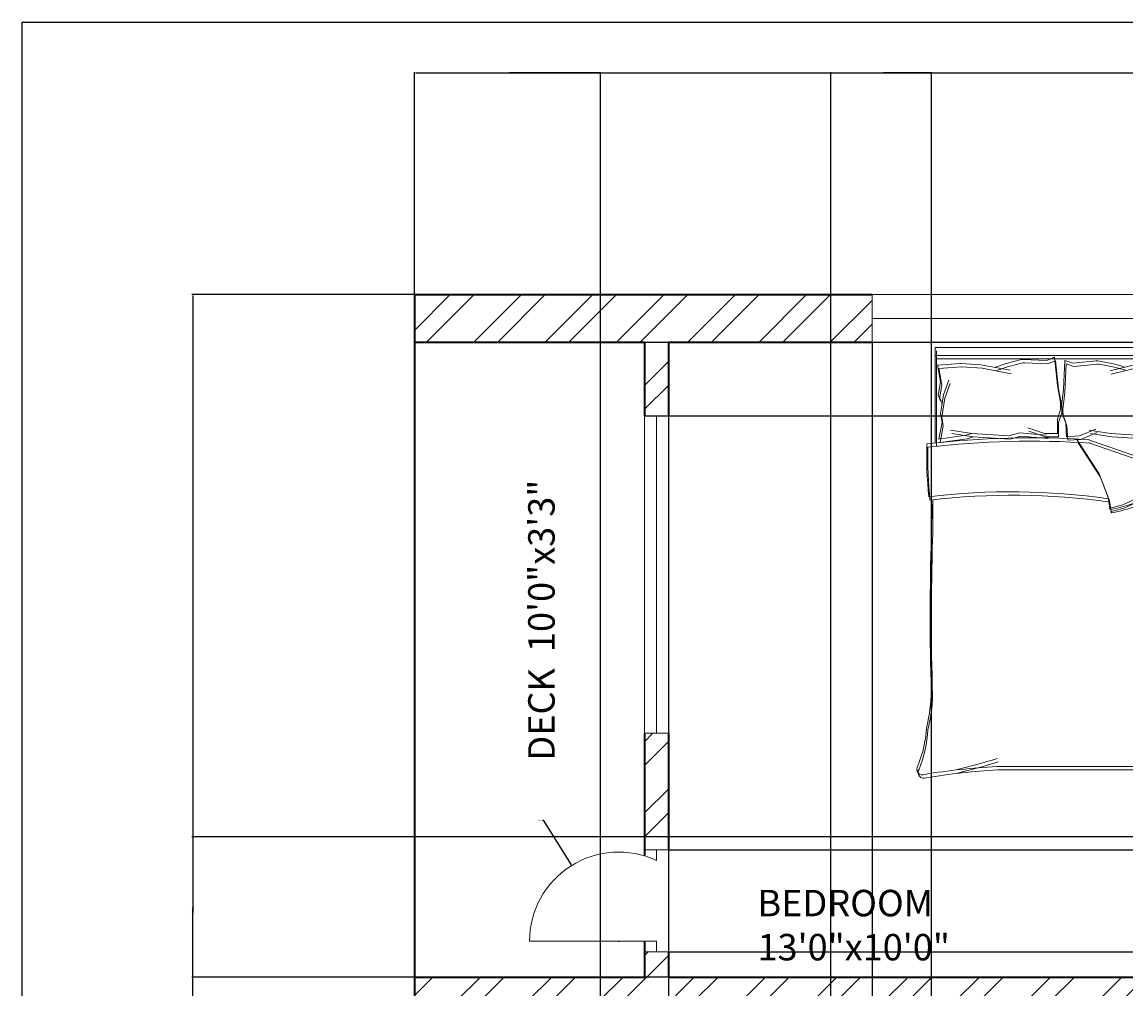
# Model space of a CAD drawing. Units: inches. Extents: x 1748 to 2382, y 1346 to 2284.
# Tile 20 of 26: x 1748 to 1956, y 2102 to 2284. Entities that reach past the tile are written whole.
import ezdxf

# ---------------------------------------------------------------- set-up
doc = ezdxf.new("R2010")
doc.units = ezdxf.units.IN
for name, color, linetype, lineweight in [('A-ANNO-DIMS', 2, 'Continuous', 18), ('A-ANNO-TTLB', 7, 'Continuous', 25), ('A-AREA-IDEN', 7, 'Continuous', 18), ('A-DOOR', 21, 'Continuous', 18), ('A-FURN', 8, 'Continuous', 13), ('A-GLAZ', 191, 'Continuous', 18), ('A-WALL', 7, 'Continuous', 35), ('A-WALL-PATT', 9, 'Continuous', 13)]:
    doc.layers.add(name, color=color, linetype=linetype, lineweight=lineweight)
doc.styles.get("Standard").update_dxf_attribs({"font": 'arial.ttf'})
doc.dimstyles.get("Standard").update_dxf_attribs({"dimtxt": 0.18, "dimasz": 0.18, "dimexe": 0.18, "dimexo": 0.0625, "dimgap": 0.09, "dimtad": 0, "dimtih": 1, "dimtoh": 1, "dimdec": 4, "dimzin": 0, "dimdsep": 46, "dimtxsty": 'Standard', "dimcen": 0.09, "dimadec": 0, "dimazin": 0, "dimtfac": 1, "dimtdec": 4, "dimtofl": 0, "dimtmove": 0, "dimatfit": 3, "dimfxl": 1, "dimtolj": 1, "dimtzin": 0, "dimarcsym": 0})

# ---------------------------------------------------------------- blocks, each defined once
blk = doc.blocks.new('BED-DOUBLE')
for p, q in [((3.48, 63.33), (3.48, 81.44)), ((3.48, 63.33), (3.48, 81.44)), ((3.48, 81.44), (51.49, 81.44)), ((51.27, 81.44), (51.27, 54.83)), ((51.27, 81.44), (51.27, 54.83)), ((51.49, 81.44), (51.49, 80.8)), ((3.48, 79.91), (51.27, 79.91)), ((3.48, 79.91), (51.27, 79.91)), ((3.7, 62.69), (3.7, 80.8)), ((3.7, 62.69), (3.7, 80.8)), ((24.54, 78.99), (25.98, 79.57)), ((24.54, 78.99), (25.98, 79.57)), ((25.98, 79.57), (26.56, 74.22)), ((25.98, 79.57), (26.56, 74.22)), ((51.49, 80.8), (51.49, 54.19)), ((51.49, 80.8), (51.49, 54.19)), ((3.7, 79.27), (51.49, 79.27)), ((3.7, 79.27), (51.49, 79.27)), ((3.89, 78.13), (4.47, 74.95)), ((3.9, 78.11), (8.18, 78.43)), ((3.9, 78.11), (8.18, 78.43)), ((3.9, 78.13), (4.47, 74.95)), ((4.12, 77.49), (4.7, 74.31)), ((4.12, 77.49), (4.7, 74.31)), ((4.13, 77.47), (8.41, 77.8)), ((4.13, 77.47), (8.41, 77.8)), ((8.18, 78.43), (8.29, 78.42)), ((8.18, 78.43), (8.28, 78.42)), ((8.28, 78.42), (12.11, 78.13)), ((8.29, 78.42), (12.11, 78.13)), ((8.41, 77.8), (8.51, 77.78)), ((8.41, 77.8), (8.51, 77.78)), ((8.51, 77.78), (12.34, 77.49)), ((8.51, 77.78), (12.34, 77.49)), ((12.11, 78.13), (17.6, 77.12)), ((12.11, 78.13), (17.6, 77.12)), ((12.34, 77.49), (17.83, 76.48)), ((12.34, 77.49), (17.83, 76.48)), ((14.86, 77.69), (16.88, 78.42)), ((14.86, 77.69), (16.88, 78.42)), ((15.08, 77.05), (17.11, 77.78)), ((15.08, 77.05), (17.11, 77.78)), ((16.88, 78.42), (19.77, 79.14)), ((16.88, 78.42), (19.77, 79.14)), ((17.11, 77.78), (20, 78.5)), ((17.11, 77.78), (20, 78.5)), ((19.77, 79.14), (20.09, 79.14)), ((19.77, 79.14), (20.09, 79.14)), ((20, 78.5), (20.32, 78.5)), ((20, 78.5), (20.32, 78.5)), ((20.09, 79.14), (24.54, 78.99)), ((20.09, 79.14), (24.54, 78.99)), ((20.32, 78.5), (24.77, 78.36)), ((20.32, 78.5), (24.77, 78.36)), ((24.77, 78.36), (26.21, 78.93)), ((24.77, 78.36), (26.21, 78.93)), ((26.21, 78.93), (26.79, 73.58)), ((26.21, 78.93), (26.79, 73.58)), ((27.98, 78.95), (27.73, 73.58)), ((27.98, 78.95), (27.73, 73.58)), ((28.21, 78.31), (27.96, 72.94)), ((28.21, 78.31), (27.96, 72.94)), ((29.46, 78.46), (27.98, 78.95)), ((29.46, 78.46), (27.98, 78.95)), ((29.68, 77.83), (28.21, 78.31)), ((29.68, 77.83), (28.21, 78.31)), ((33.88, 78.89), (29.46, 78.46)), ((33.88, 78.89), (29.46, 78.46)), ((34.11, 78.25), (29.68, 77.83)), ((34.11, 78.25), (29.68, 77.83)), ((34.21, 78.91), (33.88, 78.89)), ((34.2, 78.91), (33.88, 78.89)), ((34.43, 78.27), (34.11, 78.25)), ((34.43, 78.27), (34.11, 78.25)), ((37.14, 78.37), (34.2, 78.91)), ((37.14, 78.37), (34.21, 78.91)), ((37.36, 77.73), (34.43, 78.27)), ((37.36, 77.73), (34.43, 78.27)), ((41.91, 78.37), (36.5, 77.02)), ((41.91, 78.37), (36.5, 77.02)), ((42.14, 77.73), (36.72, 76.38)), ((42.14, 77.73), (36.72, 76.38)), ((39.2, 77.77), (37.14, 78.37)), ((39.2, 77.77), (37.14, 78.37)), ((39.43, 77.13), (37.36, 77.73)), ((39.43, 77.13), (37.36, 77.73)), ((45.71, 78.9), (41.91, 78.37)), ((45.71, 78.9), (41.91, 78.37)), ((45.94, 78.26), (42.14, 77.73)), ((45.94, 78.26), (42.14, 77.73)), ((50.11, 78.89), (44.71, 78.98)), ((44.71, 78.98), (45.71, 78.9)), ((50.11, 78.89), (44.71, 78.98)), ((44.71, 78.98), (45.71, 78.9)), ((50.34, 78.25), (44.94, 78.34)), ((44.94, 78.34), (45.94, 78.26)), ((50.34, 78.25), (44.94, 78.34)), ((44.94, 78.34), (45.94, 78.26)), ((50.11, 78.89), (49.73, 75.68)), ((50.11, 78.89), (49.73, 75.68)), ((50.34, 78.25), (49.96, 75.04)), ((50.34, 78.25), (49.96, 75.04)), ((5.05, 72.49), (6.06, 75.24)), ((5.05, 72.49), (6.06, 75.24)), ((49.31, 73.19), (48.13, 75.87)), ((49.31, 73.19), (48.13, 75.87)), ((49.54, 72.55), (48.36, 75.23)), ((49.54, 72.55), (48.36, 75.23)), ((49.73, 75.68), (50.33, 73.11)), ((49.73, 75.68), (50.33, 73.11)), ((4.47, 74.95), (4.04, 72.34)), ((4.47, 74.95), (4.04, 72.34)), ((4.7, 74.31), (4.27, 71.7)), ((4.7, 74.31), (4.27, 71.7)), ((5.28, 71.85), (6.29, 74.6)), ((5.28, 71.85), (6.29, 74.6)), ((26.56, 74.22), (27.14, 71.04)), ((26.56, 74.22), (27.14, 71.04)), ((26.79, 73.58), (27.37, 70.4)), ((26.79, 73.58), (27.37, 70.4)), ((27.73, 73.58), (27.35, 70.37)), ((27.73, 73.58), (27.36, 70.37)), ((50.11, 69.61), (49.31, 73.19)), ((50.11, 69.61), (49.31, 73.19)), ((50.33, 73.11), (49.81, 72.06)), ((50.33, 73.11), (49.81, 72.06)), ((49.96, 75.04), (50.56, 72.47)), ((49.96, 75.04), (50.56, 72.47)), ((4.04, 72.34), (4.62, 71.33)), ((4.04, 72.34), (4.62, 71.33)), ((4.27, 71.7), (4.85, 70.69)), ((4.27, 71.7), (4.85, 70.69)), ((4.47, 68.87), (5.05, 72.49)), ((4.47, 68.87), (5.05, 72.49)), ((4.7, 68.23), (5.28, 71.85)), ((4.7, 68.23), (5.28, 71.85)), ((27.14, 71.04), (27.14, 69.74)), ((27.14, 71.04), (27.14, 69.74)), ((27.96, 72.94), (27.58, 69.73)), ((27.96, 72.94), (27.58, 69.73)), ((50.34, 68.98), (49.54, 72.55)), ((50.34, 68.98), (49.54, 72.55)), ((50.56, 72.47), (50.04, 71.42)), ((50.56, 72.47), (50.04, 71.42)), ((4.76, 67.28), (4.47, 68.87)), ((4.76, 67.28), (4.47, 68.87)), ((27.14, 69.74), (26.56, 67.86)), ((27.14, 69.74), (26.56, 67.86)), ((27.37, 69.1), (26.79, 67.22)), ((27.37, 69.1), (26.79, 67.22)), ((27.35, 70.37), (27.44, 69.07)), ((27.36, 70.37), (27.44, 69.07)), ((27.37, 70.4), (27.37, 69.1)), ((27.37, 70.4), (27.37, 69.1)), ((27.44, 69.07), (28.13, 67.23)), ((27.44, 69.07), (28.13, 67.23)), ((27.58, 69.73), (27.66, 68.43)), ((27.58, 69.73), (27.66, 68.43)), ((49.92, 68.01), (50.11, 69.61)), ((49.92, 68.01), (50.11, 69.61)), ((50.15, 67.37), (50.34, 68.98)), ((50.15, 67.37), (50.34, 68.98)), ((4.18, 64.1), (4.76, 67.28)), ((4.18, 64.1), (4.76, 67.28)), ((4.99, 66.64), (4.7, 68.23)), ((4.99, 66.64), (4.7, 68.23)), ((26.56, 67.86), (26.56, 65.18)), ((26.56, 67.86), (26.56, 65.18)), ((26.79, 67.22), (26.79, 64.54)), ((26.79, 67.22), (26.79, 64.54)), ((27.66, 68.43), (28.36, 66.59)), ((27.66, 68.43), (28.36, 66.59)), ((28.13, 67.23), (28.3, 64.55)), ((28.13, 67.23), (28.3, 64.55)), ((50.7, 64.87), (49.92, 68.01)), ((50.7, 64.87), (49.92, 68.01)), ((50.93, 64.23), (50.15, 67.37)), ((50.93, 64.23), (50.15, 67.37)), ((9.28, 64.83), (4.18, 64.1)), ((9.28, 64.83), (4.18, 64.1)), ((4.41, 63.46), (4.99, 66.64)), ((4.41, 63.46), (4.99, 66.64)), ((6.38, 65.81), (10.41, 65.15)), ((6.38, 65.81), (10.41, 65.15)), ((6.61, 65.18), (10.64, 64.51)), ((6.61, 65.18), (10.64, 64.51)), ((10.41, 65.15), (9.28, 64.83)), ((10.41, 65.15), (9.28, 64.83)), ((10.41, 65.15), (17.42, 64.72)), ((10.41, 65.15), (17.42, 64.72)), ((17.42, 64.72), (19.38, 65.27)), ((17.42, 64.72), (19.38, 65.27)), ((19.38, 65.27), (24.52, 64.87)), ((19.38, 65.27), (24.52, 64.87)), ((24.1, 65.18), (20.96, 66.27)), ((24.1, 65.18), (20.96, 66.27)), ((24.33, 64.54), (21.19, 65.63)), ((24.33, 64.54), (21.19, 65.63)), ((26.56, 65.18), (24.1, 65.18)), ((26.56, 65.18), (24.1, 65.18)), ((28.3, 64.55), (30.75, 64.7)), ((28.3, 64.55), (30.75, 64.7)), ((28.36, 66.59), (28.53, 63.91)), ((28.36, 66.59), (28.53, 63.91)), ((30.75, 64.7), (33.82, 65.99)), ((30.75, 64.7), (33.82, 65.99)), ((30.98, 64.06), (34.05, 65.35)), ((30.98, 64.06), (34.05, 65.35)), ((32.56, 65.81), (36.6, 65.15)), ((32.56, 65.81), (36.6, 65.15)), ((32.79, 65.18), (36.83, 64.51)), ((32.79, 65.18), (36.82, 64.51)), ((36.6, 65.15), (43.61, 64.72)), ((36.6, 65.15), (43.61, 64.72)), ((43.61, 64.72), (45.57, 65.27)), ((43.61, 64.72), (45.57, 65.27)), ((45.57, 65.27), (50.7, 64.87)), ((45.57, 65.27), (50.7, 64.87)), ((9.51, 64.19), (4.41, 63.46)), ((9.51, 64.19), (4.41, 63.46)), ((10.64, 64.51), (9.51, 64.19)), ((10.64, 64.51), (9.51, 64.19)), ((10.64, 64.51), (17.65, 64.08)), ((10.64, 64.51), (17.65, 64.08)), ((17.65, 64.08), (19.61, 64.64)), ((17.65, 64.08), (19.61, 64.64)), ((19.61, 64.64), (24.74, 64.23)), ((19.61, 64.64), (24.74, 64.23)), ((26.79, 64.54), (24.33, 64.54)), ((26.79, 64.54), (24.33, 64.54)), ((28.53, 63.91), (30.98, 64.06)), ((28.53, 63.91), (30.98, 64.06)), ((30.26, 64.06), (34.45, 57.57)), ((30.26, 64.06), (34.45, 57.57)), ((30.49, 63.42), (34.68, 56.93)), ((30.49, 63.42), (34.68, 56.93)), ((40.64, 61.13), (32.31, 64.06)), ((40.64, 61.13), (32.31, 64.06)), ((40.87, 60.49), (32.53, 63.42)), ((40.87, 60.49), (32.53, 63.42)), ((36.82, 64.51), (43.83, 64.08)), ((36.83, 64.51), (43.83, 64.08)), ((43.83, 64.08), (45.8, 64.64)), ((43.83, 64.08), (45.79, 64.64)), ((45.79, 64.64), (50.93, 64.23)), ((45.8, 64.64), (50.93, 64.23)), ((46.22, 59.11), (40.64, 61.13)), ((46.22, 59.11), (40.64, 61.13)), ((46.45, 58.48), (40.87, 60.49)), ((46.45, 58.48), (40.87, 60.49)), ((49.16, 56.95), (46.22, 59.11)), ((49.16, 56.95), (46.22, 59.11)), ((49.39, 56.31), (46.45, 58.48)), ((49.39, 56.31), (46.45, 58.48)), ((34.45, 57.57), (36.15, 53.08)), ((34.45, 57.57), (36.15, 53.08)), ((34.68, 56.93), (36.38, 52.44)), ((34.68, 56.93), (36.38, 52.44)), ((52.87, 53.7), (49.16, 56.95)), ((52.87, 53.7), (49.16, 56.95)), ((53.1, 53.06), (49.39, 56.31)), ((53.1, 53.06), (49.39, 56.31)), ((36.15, 53.08), (36.46, 51.07)), ((36.15, 53.08), (36.46, 51.07)), ((36.38, 52.44), (36.69, 50.43)), ((36.38, 52.44), (36.69, 50.43)), ((38.94, 51.69), (40.95, 52.61)), ((38.94, 51.69), (40.95, 52.61)), ((40.95, 52.61), (44.36, 53.08)), ((40.95, 52.61), (44.36, 53.08)), ((41.18, 51.97), (44.59, 52.44)), ((41.18, 51.97), (44.59, 52.44)), ((44.36, 53.08), (48.23, 53.39)), ((44.36, 53.08), (48.23, 53.39)), ((44.59, 52.44), (48.46, 52.75)), ((44.59, 52.44), (48.46, 52.75)), ((48.23, 53.39), (51.33, 53.08)), ((48.23, 53.39), (51.33, 53.08)), ((48.46, 52.75), (51.56, 52.44)), ((48.46, 52.75), (51.56, 52.44)), ((51.33, 53.08), (52.87, 53.7)), ((51.33, 53.08), (52.87, 53.7)), ((51.56, 52.44), (53.1, 53.06)), ((51.56, 52.44), (53.1, 53.06)), ((52.95, 51.95), (52.87, 53.7, 3.87)), ((52.95, 51.95), (52.87, 53.7, 3.87)), ((53.18, 51.31), (53.1, 53.06, 3.87)), ((53.18, 51.31), (53.1, 53.06, 3.87)), ((36.46, 51.07), (38.94, 51.69)), ((36.46, 51.07), (38.94, 51.69)), ((36.69, 50.43), (39.17, 51.05)), ((36.69, 50.43), (39.17, 51.05)), ((39.17, 51.05), (41.18, 51.97)), ((39.17, 51.05), (41.18, 51.97)), ((15.06, 2.2), (39.68, 2.2)), ((15.06, 2.2), (39.68, 2.2)), ((15.29, 1.56), (39.91, 1.56)), ((15.29, 1.56), (39.91, 1.56))]:
    blk.add_line(p, q)
for centre, radius, start, end in [((85.16, 61.35), 83.31, 178.7218, 185.604), ((85.16, 61.35), 83.31, 178.7218, 185.604), ((21.36, -100.61), 164.97, 86.0865, 96.7821), ((21.36, -100.61), 164.97, 86.0865, 96.7821), ((21.59, -101.25), 164.97, 86.0865, 96.7821), ((21.59, -101.25), 164.97, 86.0865, 96.7821), ((85.39, 60.71), 83.31, 178.7218, 185.604), ((85.39, 60.71), 83.31, 178.7218, 185.604), ((17.76, -74.87), 129.02, 81.7845, 96.9006), ((17.76, -74.87), 129.02, 81.7845, 96.9006), ((17.98, -75.51), 129.02, 81.7845, 96.9006), ((17.98, -75.51), 129.02, 81.7845, 96.9006), ((-167.31, 50.27), 170.11, 358.4762, 1.0082), ((-167.31, 50.27), 170.11, 358.4762, 1.0082), ((-167.08, 49.63), 170.11, 358.4762, 1.0082), ((-167.08, 49.63), 170.11, 358.4762, 1.0082), ((43.74, 46.38), 6.22, 78.6608, 113.7384), ((43.74, 46.38), 6.22, 78.6608, 113.7384), ((51.33, 88.1), 36.18, 259.8763, 272.5657), ((51.33, 88.1), 36.18, 259.8763, 272.5657), ((36.64, 51), 0.185, 160.2464, 271.1377), ((36.64, 51), 0.185, 160.2464, 271.1377), ((31.15, 79.96), 29.65, 280.6617, 289.8806), ((31.15, 79.96), 29.65, 280.6617, 289.8806), ((36.87, 50.36), 0.185, 160.2464, 271.1377), ((36.86, 50.36), 0.185, 160.2464, 271.1377), ((31.38, 79.32), 29.65, 280.6617, 289.8806), ((31.38, 79.32), 29.65, 280.6617, 289.8806), ((43.97, 45.74), 6.22, 78.6608, 113.7384), ((43.97, 45.74), 6.22, 78.6608, 113.7384), ((51.56, 87.46), 36.18, 259.8763, 272.5657), ((51.56, 87.46), 36.18, 259.8763, 272.5657), ((182.27, 45.13), 129.5, 176.9791, 183.8365), ((182.27, 45.13), 129.5, 176.9791, 183.8365), ((182.49, 44.49), 129.5, 176.9791, 183.8365), ((182.49, 44.49), 129.5, 176.9791, 183.8365), ((484.82, 30.83), 482.31, 178.2277, 181.7185), ((484.82, 30.83), 482.31, 178.2277, 181.7185), ((485.05, 30.19), 482.31, 178.2277, 181.7185), ((485.05, 30.19), 482.31, 178.2277, 181.7185), ((-4508.74, 13.62), 4561.86, 0.00217, 0.28689), ((-4508.74, 13.62), 4561.86, 0.00217, 0.28689), ((-4508.51, 12.98), 4561.86, 0.00217, 0.28689), ((-4508.51, 12.98), 4561.86, 0.00217, 0.28689), ((-26.9, 16.93), 29.63, 346.0648, 358.9113), ((-26.9, 16.93), 29.63, 346.0648, 358.9113), ((-26.67, 16.29), 29.63, 346.0648, 358.9113), ((-26.67, 16.29), 29.63, 346.0648, 358.9113), ((76.16, 12.78), 23.07, 177.4714, 206.4681), ((76.16, 12.78), 23.07, 177.4714, 206.4681), ((76.39, 12.14), 23.07, 177.4714, 206.4681), ((76.39, 12.14), 23.07, 177.4714, 206.4681), ((-21.66, 11.17), 23.56, 337.9751, 356.652), ((-21.66, 11.17), 23.56, 337.9751, 356.652), ((-21.43, 10.53), 23.56, 337.9751, 356.652), ((-21.43, 10.53), 23.56, 337.9751, 356.652), ((1.09, 1.73), 1.09, 146.1736, 293.4781), ((1.09, 1.73), 1.09, 146.1736, 293.4781), ((21.43, -119.39), 121.76, 92.9958, 99.4091), ((21.43, -119.39), 121.76, 92.9958, 99.4091), ((-17.22, 105.16), 106.46, 283.3832, 287.7053), ((-17.22, 105.16), 106.46, 283.3832, 287.7053), ((-16.99, 104.52), 106.46, 283.3832, 287.7053), ((-16.99, 104.52), 106.46, 283.3832, 287.7053), ((41.15, -130.83), 133.04, 84.4998, 90.6351), ((41.15, -130.83), 133.04, 84.4998, 90.6351), ((54.41, 2.57), 1.1, 242.6588, 356.02), ((54.41, 2.57), 1.1, 242.6588, 356.02), ((1.32, 1.09), 1.09, 146.1736, 293.4781), ((1.32, 1.09), 1.09, 146.1736, 293.4781), ((21.66, -120.03), 121.76, 92.9958, 99.4091), ((21.66, -120.03), 121.76, 92.9958, 99.4091), ((41.38, -131.47), 133.04, 84.4998, 90.6351), ((41.38, -131.47), 133.04, 84.4998, 90.6351), ((54.64, 1.93), 1.1, 242.6588, 356.02), ((54.64, 1.93), 1.1, 242.6588, 356.02)]:
    blk.add_arc(centre, radius, start, end)
blk = doc.blocks.new('WIN-60-DEEP')
for p, q in [((0, 9), (0, 0)), ((60, 9), (0, 9)), ((60, 4.5), (60, 9)), ((60, 9), (60, 0)), ((0, 0), (0, 4.5)), ((0, 4.5), (60, 4.5)), ((0, 0), (60, 0))]:
    blk.add_line(p, q)
blk = doc.blocks.new('WIN-60-SHALLOW')
for p, q in [((0, 60), (4.5, 60)), ((0, 60), (0, 0)), ((4.5, 60), (2.25, 60)), ((2.25, 60), (2.25, 0)), ((4.5, 60), (4.5, 0)), ((2.25, 0), (0, 0)), ((0, 0), (4.5, 0))]:
    blk.add_line(p, q)
blk = doc.blocks.new('*D34')
at = {"layer": 'A-ANNO-DIMS', "color": 0, "lineweight": -2, "transparency": 16777216}
for p, q in [((1821.96, 2232.91), (1821.96, 2274.93)), ((1822.14, 2274.75), (2059.31, 2274.75)), ((2297.28, 2274.75), (2060.11, 2274.75)), ((2297.46, 2232.91), (2297.46, 2274.93))]:
    blk.add_line(p, q, dxfattribs=at)
at = {"layer": 'A-ANNO-DIMS', "color": 0, "transparency": 16777216}
for points in [[(1822.14, 2274.78), (1822.14, 2274.72), (1821.96, 2274.75)], [(2297.28, 2274.78), (2297.28, 2274.72), (2297.46, 2274.75)]]:
    blk.add_solid(points, dxfattribs=at)
at = {"layer": 'Defpoints', "color": 0, "transparency": 16777216}
for p in [(2297.46, 2274.75), (1821.96, 2232.85), (2297.46, 2232.85)]:
    blk.add_point(p, dxfattribs=at)
at = {"layer": 'A-ANNO-DIMS', "color": 0, "transparency": 16777216, "insert": (2059.71, 2274.75), "char_height": 0.18, "attachment_point": 5}
blk.add_mtext('\\A1;475.5', dxfattribs=at)
blk = doc.blocks.new('*D41')
at = {"layer": 'A-ANNO-DIMS', "color": 0, "lineweight": -2, "transparency": 16777216}
for p, q in [((1821.96, 1854.91), (1821.96, 2274.93)), ((1822.14, 2274.75), (1839.16, 2274.75)), ((1856.96, 2274.75), (1839.95, 2274.75)), ((1857.14, 1854.91), (1857.14, 2274.93))]:
    blk.add_line(p, q, dxfattribs=at)
at = {"layer": 'A-ANNO-DIMS', "color": 0, "transparency": 16777216}
for points in [[(1822.14, 2274.78), (1822.14, 2274.72), (1821.96, 2274.75)], [(1856.96, 2274.78), (1856.96, 2274.72), (1857.14, 2274.75)]]:
    blk.add_solid(points, dxfattribs=at)
at = {"layer": 'Defpoints', "color": 0, "transparency": 16777216}
for p in [(1857.14, 2274.75), (1821.96, 1854.85), (1857.14, 1854.85)]:
    blk.add_point(p, dxfattribs=at)
at = {"layer": 'A-ANNO-DIMS', "color": 0, "transparency": 16777216, "insert": (1839.55, 2274.75), "char_height": 0.18, "attachment_point": 5}
blk.add_mtext('\\A1;35.18', dxfattribs=at)
blk = doc.blocks.new('*D45')
at = {"layer": 'A-ANNO-DIMS', "color": 0, "lineweight": -2, "transparency": 16777216}
for p, q in [((1821.9, 2232.85), (1779.88, 2232.85)), ((1780.06, 2232.67), (1780.06, 2116.07)), ((1780.06, 1999.11), (1780.06, 2115.71)), ((1865.4, 1998.93), (1779.88, 1998.93))]:
    blk.add_line(p, q, dxfattribs=at)
at = {"layer": 'A-ANNO-DIMS', "color": 0, "transparency": 16777216}
for points in [[(1780.03, 2232.67), (1780.09, 2232.67), (1780.06, 2232.85)], [(1780.03, 1999.11), (1780.09, 1999.11), (1780.06, 1998.93)]]:
    blk.add_solid(points, dxfattribs=at)
at = {"layer": 'Defpoints', "color": 0, "transparency": 16777216}
for p in [(1780.06, 2232.85), (1821.96, 2232.85), (1865.46, 1998.93)]:
    blk.add_point(p, dxfattribs=at)
at = {"layer": 'A-ANNO-DIMS', "color": 0, "transparency": 16777216, "insert": (1780.06, 2115.89), "char_height": 0.18, "attachment_point": 5}
blk.add_mtext('\\A1;233.9', dxfattribs=at)
blk = doc.blocks.new('*D50')
at = {"layer": 'A-ANNO-DIMS', "color": 0, "lineweight": -2, "transparency": 16777216}
for p, q in [((1869.96, 2223.79), (1869.96, 1360.47)), ((1908.44, 2223.79), (1908.44, 1360.47)), ((1870.14, 1360.65), (1888.81, 1360.65)), ((1908.26, 1360.65), (1889.6, 1360.65))]:
    blk.add_line(p, q, dxfattribs=at)
at = {"layer": 'A-ANNO-DIMS', "color": 0, "transparency": 16777216}
for points in [[(1870.14, 1360.68), (1870.14, 1360.62), (1869.96, 1360.65)], [(1908.26, 1360.68), (1908.26, 1360.62), (1908.44, 1360.65)]]:
    blk.add_solid(points, dxfattribs=at)
at = {"layer": 'Defpoints', "color": 0, "transparency": 16777216}
for p in [(1869.96, 2223.85), (1908.44, 2223.85), (1908.44, 1360.65)]:
    blk.add_point(p, dxfattribs=at)
at = {"layer": 'A-ANNO-DIMS', "color": 0, "transparency": 16777216, "insert": (1889.2, 1360.65), "char_height": 0.18, "attachment_point": 5}
blk.add_mtext('\\A1;38.48', dxfattribs=at)
blk = doc.blocks.new('*D64')
at = {"layer": 'A-ANNO-DIMS', "color": 0, "lineweight": -2, "transparency": 16777216}
for p, q in [((1900.64, 1476.91), (1900.64, 2274.93)), ((1900.82, 2274.75), (1909.7, 2274.75)), ((1919.5, 2274.75), (1910.62, 2274.75)), ((1919.68, 1476.91), (1919.68, 2274.93))]:
    blk.add_line(p, q, dxfattribs=at)
at = {"layer": 'A-ANNO-DIMS', "color": 0, "transparency": 16777216}
for points in [[(1900.82, 2274.78), (1900.82, 2274.72), (1900.64, 2274.75)], [(1919.5, 2274.78), (1919.5, 2274.72), (1919.68, 2274.75)]]:
    blk.add_solid(points, dxfattribs=at)
at = {"layer": 'Defpoints', "color": 0, "transparency": 16777216}
for p in [(1919.68, 2274.75), (1900.64, 1476.85), (1919.68, 1476.85)]:
    blk.add_point(p, dxfattribs=at)
at = {"layer": 'A-ANNO-DIMS', "color": 0, "transparency": 16777216, "insert": (1910.16, 2274.75), "char_height": 0.18, "attachment_point": 5}
blk.add_mtext('\\A1;19.035', dxfattribs=at)
blk = doc.blocks.new('*D68')
at = {"layer": 'A-ANNO-DIMS', "color": 0, "lineweight": -2, "transparency": 16777216}
for p, q in [((1865.52, 2223.85), (2339.54, 2223.85)), ((2339.36, 2223.67), (2339.36, 2217.07)), ((2339.36, 2210.1), (2339.36, 2216.7)), ((1865.52, 2209.92), (2339.54, 2209.92))]:
    blk.add_line(p, q, dxfattribs=at)
at = {"layer": 'A-ANNO-DIMS', "color": 0, "transparency": 16777216}
for points in [[(2339.33, 2223.67), (2339.39, 2223.67), (2339.36, 2223.85)], [(2339.33, 2210.1), (2339.39, 2210.1), (2339.36, 2209.92)]]:
    blk.add_solid(points, dxfattribs=at)
at = {"layer": 'Defpoints', "color": 0, "transparency": 16777216}
for p in [(1865.46, 2223.85), (2339.36, 2223.85), (1865.46, 2209.92)]:
    blk.add_point(p, dxfattribs=at)
at = {"layer": 'A-ANNO-DIMS', "color": 0, "transparency": 16777216, "insert": (2339.36, 2216.88), "char_height": 0.18, "attachment_point": 5}
blk.add_mtext('\\A1;13.93', dxfattribs=at)
blk = doc.blocks.new('*D75')
at = {"layer": 'A-ANNO-DIMS', "color": 0, "lineweight": -2, "transparency": 16777216}
for p, q in [((2078.4, 2130.35), (1779.88, 2130.35)), ((1780.06, 2130.17), (1780.06, 2117.28)), ((1780.06, 2104.03), (1780.06, 2116.92)), ((2078.4, 2103.85), (1779.88, 2103.85))]:
    blk.add_line(p, q, dxfattribs=at)
at = {"layer": 'A-ANNO-DIMS', "color": 0, "transparency": 16777216}
for points in [[(1780.03, 2130.17), (1780.09, 2130.17), (1780.06, 2130.35)], [(1780.03, 2104.03), (1780.09, 2104.03), (1780.06, 2103.85)]]:
    blk.add_solid(points, dxfattribs=at)
at = {"layer": 'Defpoints', "color": 0, "transparency": 16777216}
for p in [(1780.06, 2130.35), (2078.46, 2130.35), (2078.46, 2103.85)]:
    blk.add_point(p, dxfattribs=at)
at = {"layer": 'A-ANNO-DIMS', "color": 0, "transparency": 16777216, "insert": (1780.06, 2117.1), "char_height": 0.18, "attachment_point": 5}
blk.add_mtext('\\A1;26.5', dxfattribs=at)
blk = doc.blocks.new('*D77')
at = {"layer": 'A-ANNO-DIMS', "color": 0, "lineweight": -2, "transparency": 16777216}
for p, q in [((1870.02, 2127.89), (2339.54, 2127.89)), ((2339.36, 2127.71), (2339.36, 2118.43)), ((2339.36, 2108.79), (2339.36, 2118.07)), ((1870.02, 2108.61), (2339.54, 2108.61))]:
    blk.add_line(p, q, dxfattribs=at)
at = {"layer": 'A-ANNO-DIMS', "color": 0, "transparency": 16777216}
for points in [[(2339.33, 2127.71), (2339.39, 2127.71), (2339.36, 2127.89)], [(2339.33, 2108.79), (2339.39, 2108.79), (2339.36, 2108.61)]]:
    blk.add_solid(points, dxfattribs=at)
at = {"layer": 'Defpoints', "color": 0, "transparency": 16777216}
for p in [(1869.96, 2127.89), (2339.36, 2127.89), (1869.96, 2108.61)]:
    blk.add_point(p, dxfattribs=at)
at = {"layer": 'A-ANNO-DIMS', "color": 0, "transparency": 16777216, "insert": (2339.36, 2118.25), "char_height": 0.18, "attachment_point": 5}
blk.add_mtext('\\A1;19.288', dxfattribs=at)
blk = doc.blocks.new('*D98')
at = {"layer": 'A-ANNO-DIMS', "color": 0, "lineweight": -2, "transparency": 16777216}
for p, q in [((1846.14, 2133.52), (1846.32, 2133.52)), ((1846.32, 2133.52), (1851.57, 2125.08)), ((1860.49, 2110.61), (1860.67, 2110.61)), ((1860.58, 2110.52), (1860.58, 2110.7))]:
    blk.add_line(p, q, dxfattribs=at)
at = {"layer": 'A-ANNO-DIMS', "color": 0, "transparency": 16777216}
blk.add_solid([(1851.6, 2125.1), (1851.55, 2125.07), (1851.67, 2124.93)], dxfattribs=at)
at = {"layer": 'Defpoints', "color": 0, "transparency": 16777216}
for p in [(1851.67, 2124.93), (1860.58, 2110.61)]:
    blk.add_point(p, dxfattribs=at)
at = {"layer": 'A-ANNO-DIMS', "color": 0, "transparency": 16777216, "insert": (1845.66, 2133.52), "char_height": 0.18, "attachment_point": 5}
blk.add_mtext('\\A1;R16.87', dxfattribs=at)

msp = doc.modelspace()

# ---------------------------------------------------------------- hatches: boundary and pattern name
at = {"layer": 'A-WALL-PATT'}
h = msp.add_hatch(dxfattribs=at)
h.set_pattern_fill('ANSI32', color=256)
h.paths.add_polyline_path([(1908.4445, 2232.8497), (1821.9607, 2232.8497), (1821.9607, 2223.8497), (1865.4607, 2223.8497), (1865.4607, 2209.9185), (1869.9607, 2209.9185), (1869.9607, 2223.8497), (1908.4445, 2223.8497), (1908.4445, 2228.3497)])
h.paths.add_polyline_path([(2040.0683, 2232.8497), (1968.4445, 2232.8497), (1968.4445, 2223.8497), (2025.9607, 2223.8497), (2025.9607, 2130.3497), (2032.1341, 2130.3497), (2032.1341, 2132.5997), (2032.1341, 2134.8497), (2030.4607, 2134.8497), (2030.4607, 2223.8497), (2040.0683, 2223.8497)])
h.paths.add_polyline_path([(2091.3969, 2232.8497), (2064.0683, 2232.8497), (2064.0683, 2223.8497), (2078.4607, 2223.8497), (2078.4607, 2134.8497), (2051.1563, 2134.8497), (2051.1563, 2130.3497), (2078.4607, 2130.3497), (2078.4607, 2128.6813), (2082.9607, 2128.6813), (2082.9607, 2130.3497), (2086.1879, 2130.3497), (2086.1879, 2132.5997), (2086.1879, 2134.8497), (2082.9607, 2134.8497), (2082.9607, 2223.8497), (2091.3969, 2223.8497), (2091.3969, 2228.3497)])
h.paths.add_polyline_path([(2167.0164, 2232.8497), (2115.3969, 2232.8497), (2115.3969, 2223.8497), (2130.9607, 2223.8497), (2130.9607, 2134.8497), (2106.9607, 2134.8497), (2106.9607, 2130.3497), (2135.4607, 2130.3497), (2135.4607, 2223.8497), (2167.0164, 2223.8497), (2167.0164, 2228.3497)])
h.paths.add_polyline_path([(1869.9607, 2149.9185), (1865.4607, 2149.9185), (1865.4607, 2127.8942), (1869.9607, 2127.8942)])
h.paths.add_polyline_path([(2082.9607, 2104.4871), (2080.7107, 2104.4871), (2078.4607, 2104.4871), (2078.4607, 2103.8497), (1869.9607, 2103.8497), (1869.9607, 2108.6062), (1867.7107, 2108.6062), (1865.4607, 2108.6062), (1865.4607, 2103.8497), (1821.9607, 2103.8497), (1821.9607, 2099.3497), (1865.4607, 2099.3497), (1865.4607, 2094.7509), (1869.9607, 2094.7509), (1869.9607, 2099.3497), (2025.9607, 2099.3497), (2025.9607, 2096.4326), (2030.4607, 2096.4326), (2030.4607, 2099.3497), (2082.9607, 2099.3497)])
h.paths.add_polyline_path([(1928.9457, 1401.1212), (2176.8693, 1401.1212), (2176.8693, 1438.214), (1928.9457, 1438.214)], flags=9)
h.paths.add_polyline_path([(2122.2668, 2048.1927), (2177.9387, 2048.1927), (2177.9387, 2066.85), (2122.2668, 2066.85)], flags=9)
h.paths.add_polyline_path([(2272.688, 2153.8197), (2272.688, 2216.746), (2262.3845, 2216.746), (2262.3845, 2153.8197)], flags=9)
h.paths.add_polyline_path([(2157.2928, 2166.5593), (2196.3822, 2166.5593), (2196.3822, 2185.2167), (2157.2928, 2185.2167)], flags=9)
h.paths.add_polyline_path([(2089.3407, 2162.0698), (2124.3987, 2162.0698), (2124.3987, 2180.7272), (2089.3407, 2180.7272)], flags=9)
h.paths.add_polyline_path([(2037.4521, 2160.0913), (2072.5101, 2160.0913), (2072.5101, 2178.7486), (2037.4521, 2178.7486)], flags=9)
h.paths.add_polyline_path([(1884.7894, 2104.1554), (1923.6297, 2104.1554), (1923.6297, 2122.8127), (1884.7894, 2122.8127)], flags=9)
h.paths.add_polyline_path([(1851.2832, 2142.9749), (1851.2832, 2199.3051), (1840.9796, 2199.3051), (1840.9796, 2142.9749)], flags=9)
h.paths.add_polyline_path([(1844.8763, 2017.2834), (1844.8763, 2073.6136), (1834.5728, 2073.6136), (1834.5728, 2017.2834)], flags=9)
h.paths.add_polyline_path([(1897.1577, 2073.1279), (1935.9981, 2073.1279), (1935.9981, 2091.7853), (1897.1577, 2091.7853)], flags=9)
h.paths.add_polyline_path([(1952.3395, 1802.4231), (2008.0114, 1802.4231), (2008.0114, 1821.0805), (1952.3395, 1821.0805)], flags=9)
h.paths.add_polyline_path([(1978.8184, 1857.6841), (2017.7338, 1857.6841), (2017.7338, 1876.3415), (1978.8184, 1876.3415)], flags=9)
h.paths.add_polyline_path([(1979.6513, 1925.9516), (2008.8089, 1925.9516), (2008.8089, 1944.6089), (1979.6513, 1944.6089)], flags=9)
h.paths.add_polyline_path([(1838.5553, 1860.3527), (1877.3957, 1860.3527), (1877.3957, 1879.01), (1838.5553, 1879.01)], flags=9)
h.paths.add_polyline_path([(1883.9018, 1787.3013), (1883.9018, 1843.6315), (1873.5983, 1843.6315), (1873.5983, 1787.3013)], flags=9)
h.paths.add_polyline_path([(1873.7079, 1509.1938), (1873.7079, 1583.7709), (1863.4044, 1583.7709), (1863.4044, 1509.1938)], flags=9)
h.paths.add_polyline_path([(1916.2259, 1603.3681), (1955.0663, 1603.3681), (1955.0663, 1622.0254), (1916.2259, 1622.0254)], flags=9)
h.paths.add_polyline_path([(1876.3013, 1636.757), (1876.3013, 1693.0871), (1865.9978, 1693.0871), (1865.9978, 1636.757)], flags=9)
h.paths.add_polyline_path([(1921.3138, 1521.8316), (1964.0662, 1521.8316), (1964.0662, 1540.489), (1921.3138, 1540.489)], flags=9)
h.paths.add_polyline_path([(2017.5657, 1497.5078), (2046.7983, 1497.5078), (2046.7983, 1516.1651), (2017.5657, 1516.1651)], flags=9)
h.paths.add_polyline_path([(2066.8661, 1499.3902), (2096.0988, 1499.3902), (2096.0988, 1518.0475), (2066.8661, 1518.0475)], flags=9)
h.paths.add_polyline_path([(2155.4835, 1571.6596), (2198.2358, 1571.6596), (2198.2358, 1590.3169), (2155.4835, 1590.3169)], flags=9)
h.paths.add_polyline_path([(2094.9136, 1664.6812), (2150.5855, 1664.6812), (2150.5855, 1683.3386), (2094.9136, 1683.3386)], flags=9)
h.paths.add_polyline_path([(2257.6902, 1863.1628), (2269.8935, 1863.1628), (2269.8935, 1873.4664), (2257.6902, 1873.4664)], flags=9)
h.paths.add_polyline_path([(2164.0748, 1880.3089), (2189.8694, 1880.3089), (2189.8694, 1890.6124), (2164.0748, 1890.6124)], flags=9)
h.paths.add_polyline_path([(2239.4394, 1931.0585), (2268.8187, 1931.0585), (2268.8187, 1949.7159), (2239.4394, 1949.7159)], flags=9)
h = msp.add_hatch(dxfattribs=at)
h.set_pattern_fill('ANSI32', color=256)
h.paths.add_polyline_path([(2297.4607, 2232.8497), (2203.0164, 2232.8497), (2203.0164, 2223.8497), (2244.9607, 2223.8497), (2244.9607, 2127.8554), (2249.4607, 2127.8554), (2249.4607, 2223.8497), (2297.4607, 2223.8497)])
h.paths.add_polyline_path([(2297.4607, 2103.8497), (2249.4607, 2103.8497), (2249.4607, 2106.7497), (2247.2107, 2106.7497), (2244.9607, 2106.7497), (2244.9607, 2103.8497), (2130.9607, 2103.8497), (2130.9607, 2099.3497), (2288.4607, 2099.3497), (2288.4607, 2077.2008), (2297.4607, 2077.2008)])
h.paths.add_polyline_path([(1928.9457, 1401.1212), (2176.8693, 1401.1212), (2176.8693, 1438.214), (1928.9457, 1438.214)], flags=9)
h.paths.add_polyline_path([(2122.2668, 2048.1927), (2177.9387, 2048.1927), (2177.9387, 2066.85), (2122.2668, 2066.85)], flags=9)
h.paths.add_polyline_path([(2272.688, 2153.8197), (2272.688, 2216.746), (2262.3845, 2216.746), (2262.3845, 2153.8197)], flags=25)
h.paths.add_polyline_path([(2157.2928, 2166.5593), (2196.3822, 2166.5593), (2196.3822, 2185.2167), (2157.2928, 2185.2167)], flags=9)
h.paths.add_polyline_path([(2089.3407, 2162.0698), (2124.3987, 2162.0698), (2124.3987, 2180.7272), (2089.3407, 2180.7272)], flags=9)
h.paths.add_polyline_path([(2037.4521, 2160.0913), (2072.5101, 2160.0913), (2072.5101, 2178.7486), (2037.4521, 2178.7486)], flags=9)
h.paths.add_polyline_path([(1884.7894, 2104.1554), (1923.6297, 2104.1554), (1923.6297, 2122.8127), (1884.7894, 2122.8127)], flags=9)
h.paths.add_polyline_path([(1851.2832, 2142.9749), (1851.2832, 2199.3051), (1840.9796, 2199.3051), (1840.9796, 2142.9749)], flags=9)
h.paths.add_polyline_path([(1844.8763, 2017.2834), (1844.8763, 2073.6136), (1834.5728, 2073.6136), (1834.5728, 2017.2834)], flags=9)
h.paths.add_polyline_path([(1897.1577, 2073.1279), (1935.9981, 2073.1279), (1935.9981, 2091.7853), (1897.1577, 2091.7853)], flags=9)
h.paths.add_polyline_path([(1952.3395, 1802.4231), (2008.0114, 1802.4231), (2008.0114, 1821.0805), (1952.3395, 1821.0805)], flags=9)
h.paths.add_polyline_path([(1978.8184, 1857.6841), (2017.7338, 1857.6841), (2017.7338, 1876.3415), (1978.8184, 1876.3415)], flags=9)
h.paths.add_polyline_path([(1979.6513, 1925.9516), (2008.8089, 1925.9516), (2008.8089, 1944.6089), (1979.6513, 1944.6089)], flags=9)
h.paths.add_polyline_path([(1838.5553, 1860.3527), (1877.3957, 1860.3527), (1877.3957, 1879.01), (1838.5553, 1879.01)], flags=9)
h.paths.add_polyline_path([(1883.9018, 1787.3013), (1883.9018, 1843.6315), (1873.5983, 1843.6315), (1873.5983, 1787.3013)], flags=9)
h.paths.add_polyline_path([(1873.7079, 1509.1938), (1873.7079, 1583.7709), (1863.4044, 1583.7709), (1863.4044, 1509.1938)], flags=9)
h.paths.add_polyline_path([(1916.2259, 1603.3681), (1955.0663, 1603.3681), (1955.0663, 1622.0254), (1916.2259, 1622.0254)], flags=9)
h.paths.add_polyline_path([(1876.3013, 1636.757), (1876.3013, 1693.0871), (1865.9978, 1693.0871), (1865.9978, 1636.757)], flags=9)
h.paths.add_polyline_path([(1921.3138, 1521.8316), (1964.0662, 1521.8316), (1964.0662, 1540.489), (1921.3138, 1540.489)], flags=9)
h.paths.add_polyline_path([(2017.5657, 1497.5078), (2046.7983, 1497.5078), (2046.7983, 1516.1651), (2017.5657, 1516.1651)], flags=9)
h.paths.add_polyline_path([(2066.8661, 1499.3902), (2096.0988, 1499.3902), (2096.0988, 1518.0475), (2066.8661, 1518.0475)], flags=9)
h.paths.add_polyline_path([(2155.4835, 1571.6596), (2198.2358, 1571.6596), (2198.2358, 1590.3169), (2155.4835, 1590.3169)], flags=9)
h.paths.add_polyline_path([(2094.9136, 1664.6812), (2150.5855, 1664.6812), (2150.5855, 1683.3386), (2094.9136, 1683.3386)], flags=9)
h.paths.add_polyline_path([(2257.6902, 1863.1628), (2269.8935, 1863.1628), (2269.8935, 1873.4664), (2257.6902, 1873.4664)], flags=9)
h.paths.add_polyline_path([(2164.0748, 1880.3089), (2189.8694, 1880.3089), (2189.8694, 1890.6124), (2164.0748, 1890.6124)], flags=9)
h.paths.add_polyline_path([(2239.4394, 1931.0585), (2268.8187, 1931.0585), (2268.8187, 1949.7159), (2239.4394, 1949.7159)], flags=9)
h = msp.add_hatch(dxfattribs=at)
h.set_pattern_fill('ANSI32', color=256)
h.paths.add_polyline_path([(1919.6777, 1476.8497), (1900.6426, 1476.8497), (1900.6426, 1522.0826), (1898.3926, 1522.0826), (1896.1426, 1522.0826), (1896.1426, 1476.8497), (1857.1426, 1476.8497), (1857.1426, 1467.8497), (1896.1426, 1467.8497), (1919.6777, 1467.8497), (1919.6777, 1472.3497)])
h.paths.add_polyline_path([(2018.7873, 1472.3497), (2018.7873, 1476.8497), (2010.9607, 1476.8497), (2010.9607, 1560.8497), (2034.9607, 1560.8497), (2034.9607, 1565.3497), (2006.4607, 1565.3497), (2006.4607, 1476.8497), (1955.6777, 1476.8497), (1955.6777, 1467.8497), (2018.7873, 1467.8497)])
h.paths.add_polyline_path([(2152.3354, 1472.3497), (2152.3354, 1476.8497), (2115.9607, 1476.8497), (2115.9607, 1565.3497), (2109.2204, 1565.3497), (2109.2204, 1563.0997), (2109.2204, 1560.8497), (2111.4607, 1560.8497), (2111.4607, 1476.8497), (2095.3617, 1476.8497), (2095.3617, 1467.8497), (2152.3354, 1467.8497)])
h.paths.add_polyline_path([(2071.3617, 1476.8497), (2063.4607, 1476.8497), (2063.4607, 1560.8497), (2090.1865, 1560.8497), (2090.1865, 1565.3497), (2063.4607, 1565.3497), (2063.4607, 1572.5485), (2061.2107, 1572.5485), (2058.9607, 1572.5485), (2058.9607, 1565.3497), (2055.6281, 1565.3497), (2055.6281, 1560.8497), (2058.9607, 1560.8497), (2058.9607, 1476.8497), (2042.7873, 1476.8497), (2042.7873, 1467.8497), (2071.3617, 1467.8497), (2071.3617, 1472.3497)])
h.paths.add_polyline_path([(2297.4607, 1506.5652), (2288.4607, 1506.5652), (2288.4607, 1476.8497), (2212.3354, 1476.8497), (2212.3354, 1467.8497), (2297.4607, 1467.8497)])
h.paths.add_polyline_path([(2297.4607, 1645.3038), (2288.4607, 1645.3038), (2288.4607, 1605.8497), (2058.9607, 1605.8497), (2058.9607, 1600.1857), (2061.2107, 1600.1857), (2063.4607, 1600.1857), (2063.4607, 1601.3497), (2288.4607, 1601.3497), (2288.4607, 1566.5652), (2297.4607, 1566.5652)])
h.paths.add_polyline_path([(2010.9607, 1609.0561), (2008.7107, 1609.0561), (2006.4607, 1609.0561), (2006.4607, 1605.8497), (1900.6426, 1605.8497), (1900.6426, 1609.7171), (1898.3926, 1609.7171), (1896.1426, 1609.7171), (1896.1426, 1605.8497), (1857.1426, 1605.8497), (1857.1426, 1601.3497), (1896.1426, 1601.3497), (1896.1426, 1542.5447), (1900.6426, 1542.5447), (1900.6426, 1601.3497), (2010.9607, 1601.3497)])
h.paths.add_polyline_path([(1928.9457, 1401.1212), (2176.8693, 1401.1212), (2176.8693, 1438.214), (1928.9457, 1438.214)], flags=9)
h.paths.add_polyline_path([(2122.2668, 2048.1927), (2177.9387, 2048.1927), (2177.9387, 2066.85), (2122.2668, 2066.85)], flags=9)
h.paths.add_polyline_path([(2272.688, 2153.8197), (2272.688, 2216.746), (2262.3845, 2216.746), (2262.3845, 2153.8197)], flags=9)
h.paths.add_polyline_path([(2157.2928, 2166.5593), (2196.3822, 2166.5593), (2196.3822, 2185.2167), (2157.2928, 2185.2167)], flags=9)
h.paths.add_polyline_path([(2089.3407, 2162.0698), (2124.3987, 2162.0698), (2124.3987, 2180.7272), (2089.3407, 2180.7272)], flags=9)
h.paths.add_polyline_path([(2037.4521, 2160.0913), (2072.5101, 2160.0913), (2072.5101, 2178.7486), (2037.4521, 2178.7486)], flags=9)
h.paths.add_polyline_path([(1884.7894, 2104.1554), (1923.6297, 2104.1554), (1923.6297, 2122.8127), (1884.7894, 2122.8127)], flags=9)
h.paths.add_polyline_path([(1851.2832, 2142.9749), (1851.2832, 2199.3051), (1840.9796, 2199.3051), (1840.9796, 2142.9749)], flags=9)
h.paths.add_polyline_path([(1844.8763, 2017.2834), (1844.8763, 2073.6136), (1834.5728, 2073.6136), (1834.5728, 2017.2834)], flags=9)
h.paths.add_polyline_path([(1897.1577, 2073.1279), (1935.9981, 2073.1279), (1935.9981, 2091.7853), (1897.1577, 2091.7853)], flags=9)
h.paths.add_polyline_path([(1952.3395, 1802.4231), (2008.0114, 1802.4231), (2008.0114, 1821.0805), (1952.3395, 1821.0805)], flags=9)
h.paths.add_polyline_path([(1978.8184, 1857.6841), (2017.7338, 1857.6841), (2017.7338, 1876.3415), (1978.8184, 1876.3415)], flags=9)
h.paths.add_polyline_path([(1979.6513, 1925.9516), (2008.8089, 1925.9516), (2008.8089, 1944.6089), (1979.6513, 1944.6089)], flags=9)
h.paths.add_polyline_path([(1838.5553, 1860.3527), (1877.3957, 1860.3527), (1877.3957, 1879.01), (1838.5553, 1879.01)], flags=9)
h.paths.add_polyline_path([(1883.9018, 1787.3013), (1883.9018, 1843.6315), (1873.5983, 1843.6315), (1873.5983, 1787.3013)], flags=9)
h.paths.add_polyline_path([(1873.7079, 1509.1938), (1873.7079, 1583.7709), (1863.4044, 1583.7709), (1863.4044, 1509.1938)], flags=9)
h.paths.add_polyline_path([(1916.2259, 1603.3681), (1955.0663, 1603.3681), (1955.0663, 1622.0254), (1916.2259, 1622.0254)], flags=9)
h.paths.add_polyline_path([(1876.3013, 1636.757), (1876.3013, 1693.0871), (1865.9978, 1693.0871), (1865.9978, 1636.757)], flags=9)
h.paths.add_polyline_path([(1921.3138, 1521.8316), (1964.0662, 1521.8316), (1964.0662, 1540.489), (1921.3138, 1540.489)], flags=9)
h.paths.add_polyline_path([(2017.5657, 1497.5078), (2046.7983, 1497.5078), (2046.7983, 1516.1651), (2017.5657, 1516.1651)], flags=9)
h.paths.add_polyline_path([(2066.8661, 1499.3902), (2096.0988, 1499.3902), (2096.0988, 1518.0475), (2066.8661, 1518.0475)], flags=9)
h.paths.add_polyline_path([(2155.4835, 1571.6596), (2198.2358, 1571.6596), (2198.2358, 1590.3169), (2155.4835, 1590.3169)], flags=25)
h.paths.add_polyline_path([(2094.9136, 1664.6812), (2150.5855, 1664.6812), (2150.5855, 1683.3386), (2094.9136, 1683.3386)], flags=9)
h.paths.add_polyline_path([(2257.6902, 1863.1628), (2269.8935, 1863.1628), (2269.8935, 1873.4664), (2257.6902, 1873.4664)], flags=9)
h.paths.add_polyline_path([(2164.0748, 1880.3089), (2189.8694, 1880.3089), (2189.8694, 1890.6124), (2164.0748, 1890.6124)], flags=9)
h.paths.add_polyline_path([(2239.4394, 1931.0585), (2268.8187, 1931.0585), (2268.8187, 1949.7159), (2239.4394, 1949.7159)], flags=9)

# ---------------------------------------------------------------- linework, layer by layer
at = {"layer": 'A-ANNO-TTLB'}
msp.add_lwpolyline([(1747.8112, 2284.3704), (2382.1361, 2284.3704), (2382.1361, 1346.4899), (1747.8112, 1346.4899)], close=True, dxfattribs=at)
at = {"layer": 'A-DOOR'}
for p, q in [((1865.4607, 2127.8942), (1869.9607, 2127.8942)), ((1869.9607, 2127.8942), (1867.7107, 2127.8942)), ((1867.7107, 2127.8942), (1867.7107, 2125.8942)), ((1867.7107, 2110.6062), (1843.7107, 2110.6062)), ((1867.7107, 2108.6062), (1867.7107, 2110.6062)), ((1865.4607, 2108.6062), (1869.9607, 2108.6062)), ((1869.9607, 2108.6062), (1867.7107, 2108.6062))]:
    msp.add_line(p, q, dxfattribs=at)
msp.add_arc((1860.5799, 2110.6062), 16.8692, 64.994277, 180, dxfattribs=at)
at = {"layer": 'A-WALL'}
for p, q in [((1821.9607, 2232.8497), (1908.4445, 2232.8497)), ((1821.9607, 2232.8497), (1821.9607, 1952.7922)), ((1821.9607, 2223.8497), (1865.4607, 2223.8497)), ((1865.4607, 2223.8497), (1865.4607, 2209.9185)), ((1869.9607, 2223.8497), (1869.9607, 2209.9185)), ((1869.9607, 2223.8497), (1908.4445, 2223.8497)), ((1865.4607, 2149.9185), (1865.4607, 2126.754)), ((1869.9607, 2149.9185), (1869.9607, 2127.8942)), ((1865.4607, 2110.6062), (1865.4607, 2103.8497)), ((1869.9607, 2108.6062), (1869.9607, 2103.8497)), ((1821.9607, 2103.8497), (1865.4607, 2103.8497)), ((1869.9607, 2103.8497), (2078.4607, 2103.8497))]:
    msp.add_line(p, q, dxfattribs=at)

# ---------------------------------------------------------------- block references
at = {"layer": 'A-FURN'}
msp.add_blockref('BED-DOUBLE', (1916.92, 2141.426), dxfattribs=at)
at = {"layer": 'A-GLAZ', "extrusion": (0, 0, -1), "zscale": -1, "rotation": 180}
msp.add_blockref('WIN-60-DEEP', (-1908.444, 2232.8493), dxfattribs=at)
at = {"layer": 'A-GLAZ', "extrusion": (0, 0, -1), "zscale": -1}
msp.add_blockref('WIN-60-SHALLOW', (-1869.9603, 2149.9184), dxfattribs=at)

# ---------------------------------------------------------------- texts
at = {"layer": 'A-AREA-IDEN', "insert": (1843.4677, 2144.7638), "char_height": 5, "attachment_point": 1, "rotation": 90}
msp.add_mtext_dynamic_manual_height_columns('DECK  10\'0"x3\'3"', width=151.587178, gutter_width=12.5, heights=[0], dxfattribs=at)
at = {"layer": 'A-AREA-IDEN', "insert": (1886.7999, 2120.3281), "char_height": 5, "attachment_point": 1}
msp.add_mtext_dynamic_manual_height_columns('BEDROOM\\P13\'0"x10\'0"', width=134.854269, gutter_width=12.5, heights=[0], dxfattribs=at)

# ---------------------------------------------------------------- dimensions: what is measured, and where the dimension line sits
at = {"layer": 'A-ANNO-DIMS'}
for base, p1, p2, override, picture, middle in [((2297.4607, 2274.7497), (1821.9607, 2232.8497), (2297.4607, 2232.8497), {"dimdec": 1, "dimlfac": 1, "dimrnd": 0, "dimzin": 0, "dimdsep": 46, "dimlunit": 2}, '*D34', (2059.7107, 2274.7497)), ((1857.1426, 2274.7497), (1821.9607, 1854.8497), (1857.1426, 1854.8497), {"dimdec": 2, "dimlfac": 1, "dimrnd": 0, "dimzin": 0, "dimdsep": 46, "dimlunit": 2}, '*D41', (1839.5517, 2274.7497)), ((1919.6777, 2274.7497), (1900.6426, 1476.8497), (1919.6777, 1476.8497), {"dimdec": 3, "dimlfac": 1, "dimrnd": 0, "dimzin": 0, "dimdsep": 46, "dimlunit": 2}, '*D64', (1910.1602, 2274.7497)), ((1908.4445, 1360.6451), (1869.9607, 2223.8497), (1908.4445, 2223.8497), {"dimdec": 2, "dimlfac": 1, "dimrnd": 0, "dimzin": 0, "dimdsep": 46, "dimlunit": 2}, '*D50', (1889.2026, 1360.6451))]:
    dim = msp.add_linear_dim(base=base, p1=p1, p2=p2, dimstyle='Standard', override=override, dxfattribs=at)
    dim.commit()
    dim.dimension.update_dxf_attribs({"geometry": picture, "text_midpoint": middle})
for base, p1, p2, override, picture, middle in [((1780.0607, 2232.8497), (1865.4607, 1998.93), (1821.9607, 2232.8497), {"dimdec": 1, "dimlfac": 1, "dimrnd": 0, "dimzin": 0, "dimdsep": 46, "dimlunit": 2}, '*D45', (1780.0607, 2115.8898)), ((2339.3607, 2223.8497), (1865.4607, 2209.9185), (1865.4607, 2223.8497), {"dimdec": 2, "dimlfac": 1, "dimrnd": 0, "dimzin": 0, "dimdsep": 46, "dimlunit": 2}, '*D68', (2339.3607, 2216.8841)), ((1780.0607, 2130.3497), (2078.4607, 2103.8497), (2078.4607, 2130.3497), {"dimdec": 1, "dimlfac": 1, "dimrnd": 0, "dimzin": 0, "dimdsep": 46, "dimlunit": 2}, '*D75', (1780.0607, 2117.0997)), ((2339.3607, 2127.8942), (1869.9607, 2108.6062), (1869.9607, 2127.8942), {"dimdec": 3, "dimlfac": 1, "dimrnd": 0, "dimzin": 0, "dimdsep": 46, "dimlunit": 2}, '*D77', (2339.3607, 2118.2502))]:
    dim = msp.add_linear_dim(base=base, p1=p1, p2=p2, angle=90, dimstyle='Standard', override=override, dxfattribs=at)
    dim.commit()
    dim.dimension.update_dxf_attribs({"geometry": picture, "text_midpoint": middle})
dim = msp.add_radius_dim(center=(1860.5799, 2110.6062), mpoint=(1851.6668, 2124.9285), dimstyle='Standard', override={"dimdec": 2, "dimlfac": 1, "dimrnd": 0, "dimzin": 0, "dimdsep": 46, "dimlunit": 2}, dxfattribs=at)
dim.commit()
dim.dimension.update_dxf_attribs({"geometry": '*D98', "text_midpoint": (1845.6591, 2133.5219), "dimtype": 164})

doc.saveas('drawing.dxf')
